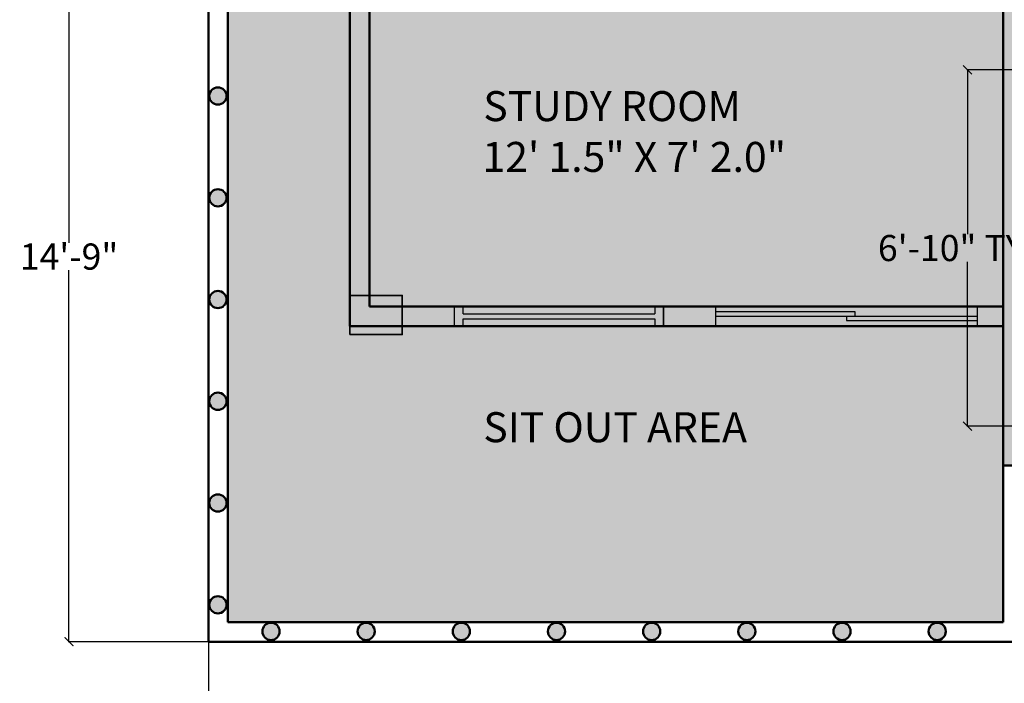
# Model space of a CAD drawing. Units: inches. Extents: x 528 to 2620, y -1066 to 798.
# Tile 21 of 41: x 981 to 1207, y 219 to 371. Entities that reach past the tile are written whole.
import ezdxf

# ---------------------------------------------------------------- set-up
doc = ezdxf.new("R2010")
doc.units = ezdxf.units.IN
doc.header["$MEASUREMENT"] = 0
for name, color, linetype, lineweight in [('A-ANNO-DIMS', 2, 'Continuous', 18), ('A-AREA-IDEN', 7, 'Continuous', 18), ('A-COLS', 1, 'Continuous', 35), ('A-Door', 2, 'Continuous', 25), ('A-GLAZ', 3, 'Continuous', 25), ('A-WALL', 7, 'Continuous', 50), ('A-WALL-PATT', 8, 'Continuous', 13)]:
    doc.layers.add(name, color=color, linetype=linetype, lineweight=lineweight)
doc.styles.get("Standard").update_dxf_attribs({"font": 'arial.ttf'})
doc.dimstyles.get("Standard").update_dxf_attribs({"dimtxt": 6, "dimasz": 2, "dimexe": 0.18, "dimexo": 0.0625, "dimgap": 0.09, "dimtad": 0, "dimtih": 1, "dimtoh": 1, "dimdec": 1, "dimzin": 0, "dimdsep": 46, "dimlunit": 3, "dimtxsty": 'Standard', "dimblk": 'ARCHTICK', "dimcen": 0.09, "dimadec": 0, "dimazin": 0, "dimtfac": 1, "dimtdec": 1, "dimtofl": 0, "dimtmove": 0, "dimatfit": 3, "dimfxl": 1, "dimtolj": 1, "dimtzin": 0, "dimarcsym": 0})

# ---------------------------------------------------------------- blocks, each defined once
blk = doc.blocks.new('_ArchTick')
at = {"color": 0, "linetype": 'ByBlock', "const_width": 0.15}
blk.add_lwpolyline([(-0.5, -0.5), (0.5, 0.5)], dxfattribs=at)
blk = doc.blocks.new('*D47')
at = {"layer": 'A-ANNO-DIMS', "color": 0, "lineweight": -2, "transparency": 16777216}
for p, q in [((1215.93, 359.77), (1198.62, 359.77)), ((1198.8, 359.77), (1198.8, 322)), ((1198.8, 277.92), (1198.8, 315.69)), ((1215.93, 277.92), (1198.62, 277.92))]:
    blk.add_line(p, q, dxfattribs=at)
at = {"layer": 'Defpoints', "color": 0, "transparency": 16777216}
for p in [(1216, 359.77), (1198.8, 277.92), (1216, 277.92)]:
    blk.add_point(p, dxfattribs=at)
at = {"layer": 'A-ANNO-DIMS', "color": 0, "lineweight": -2, "transparency": 16777216, "xscale": 2, "yscale": 2, "zscale": 2}
for p, rotation in [((1198.8, 359.77), 90), ((1198.8, 277.92), 270)]:
    blk.add_blockref('_ArchTick', p, dxfattribs=dict(at, rotation=rotation))
at = {"layer": 'A-ANNO-DIMS', "color": 0, "transparency": 16777216, "insert": (1198.8, 318.84), "char_height": 6, "attachment_point": 5}
blk.add_mtext('\\A1;6\'-10" TYP.', dxfattribs=at)
blk = doc.blocks.new('*D60')
at = {"layer": 'A-ANNO-DIMS', "color": 0, "lineweight": -2, "transparency": 16777216}
for p, q in [((1024.5, 228.36), (1024.5, 196.24)), ((1211.5, 228.36), (1211.5, 196.24)), ((1024.5, 196.42), (1107.88, 196.42)), ((1211.5, 196.42), (1128.11, 196.42))]:
    blk.add_line(p, q, dxfattribs=at)
at = {"layer": 'Defpoints', "color": 0, "transparency": 16777216}
for p in [(1024.5, 228.42), (1211.5, 228.42), (1211.5, 196.42)]:
    blk.add_point(p, dxfattribs=at)
at = {"layer": 'A-ANNO-DIMS', "color": 0, "lineweight": -2, "transparency": 16777216, "xscale": 2, "yscale": 2, "zscale": 2, "rotation": 180}
blk.add_blockref('_ArchTick', (1024.5, 196.42), dxfattribs=at)
at = {"layer": 'A-ANNO-DIMS', "color": 0, "lineweight": -2, "transparency": 16777216, "xscale": 2, "yscale": 2, "zscale": 2}
blk.add_blockref('_ArchTick', (1211.5, 196.42), dxfattribs=at)
at = {"layer": 'A-ANNO-DIMS', "color": 0, "transparency": 16777216, "insert": (1118, 196.42), "char_height": 6, "attachment_point": 5}
blk.add_mtext('\\A1;15\'-7"', dxfattribs=at)
blk = doc.blocks.new('*D64')
at = {"layer": 'A-ANNO-DIMS', "color": 0, "lineweight": -2, "transparency": 16777216}
for p, q in [((1024.43, 405.34), (992.32, 405.34)), ((992.5, 405.34), (992.5, 320.03)), ((992.5, 228.42), (992.5, 313.73)), ((1024.43, 228.42), (992.32, 228.42))]:
    blk.add_line(p, q, dxfattribs=at)
at = {"layer": 'Defpoints', "color": 0, "transparency": 16777216}
for p in [(1024.5, 405.34), (992.5, 228.42), (1024.5, 228.42)]:
    blk.add_point(p, dxfattribs=at)
at = {"layer": 'A-ANNO-DIMS', "color": 0, "lineweight": -2, "transparency": 16777216, "xscale": 2, "yscale": 2, "zscale": 2}
for p, rotation in [((992.5, 405.34), 90), ((992.5, 228.42), 270)]:
    blk.add_blockref('_ArchTick', p, dxfattribs=dict(at, rotation=rotation))
at = {"layer": 'A-ANNO-DIMS', "color": 0, "transparency": 16777216, "insert": (992.5, 316.88), "char_height": 6, "attachment_point": 5}
blk.add_mtext('\\A1;14\'-9"', dxfattribs=at)

msp = doc.modelspace()

# ---------------------------------------------------------------- hatches: boundary and pattern name
at = {"layer": 'A-COLS', "transparency": 33554687}
h = msp.add_hatch(color=256, dxfattribs=at)
h.dxf.hatch_style = 1
h.paths.add_polyline_path([(1057, 307.96), (1057, 298.96), (1069, 298.96), (1069, 307.96)])
at = {"layer": 'A-Door', "transparency": 33554687}
h = msp.add_hatch(color=256, dxfattribs=at)
h.dxf.hatch_style = 1
h.paths.add_polyline_path([(1201, 305.42), (1141, 305.42), (1141, 304.19), (1173.04, 304.19), (1173.04, 303.17), (1201, 303.17)])
h.paths.add_polyline_path([(1201, 302.21), (1171, 302.21), (1171, 303.17), (1141, 303.17), (1141, 300.92), (1201, 300.92)])
h = msp.add_hatch(color=256, dxfattribs=at)
h.dxf.hatch_style = 1
h.paths.add_polyline_path([(1201, 303.17), (1173.04, 303.17), (1171, 303.17), (1171, 302.21), (1201, 302.21)])
h.paths.add_polyline_path([(1173.04, 304.19), (1141, 304.19), (1141, 303.17), (1171, 303.17), (1173.04, 303.17)])
at = {"layer": 'A-GLAZ', "transparency": 33554687}
h = msp.add_hatch(color=256, dxfattribs=at)
h.dxf.hatch_style = 1
h.paths.add_polyline_path([(1061.5, 391.42), (1057, 391.42), (1057, 307.96), (1061.5, 307.96)])
h.paths.add_polyline_path([(1081, 305.42), (1069, 305.42), (1069, 300.92), (1081, 300.92)])
h.paths.add_polyline_path([(1141, 305.42), (1129, 305.42), (1129, 300.92), (1141, 300.92)])
h.paths.add_polyline_path([(1207, 305.42), (1201, 305.42), (1201, 300.92), (1207, 300.92)])
h = msp.add_hatch(color=256, dxfattribs=at)
h.dxf.hatch_style = 1
h.paths.add_polyline_path([(1129, 305.42), (1127, 305.42), (1127, 303.75), (1083, 303.75), (1083, 305.42), (1081, 305.42), (1081, 300.92), (1083, 300.92), (1083, 302.6), (1127, 302.6), (1127, 300.92), (1129, 300.92)])
h = msp.add_hatch(color=256, dxfattribs=at)
h.dxf.hatch_style = 1
h.paths.add_polyline_path([(1127, 305.42), (1083, 305.42), (1083, 303.75), (1127, 303.75)])
h.paths.add_polyline_path([(1127, 302.6), (1083, 302.6), (1083, 300.92), (1127, 300.92)])
at = {"layer": 'A-WALL-PATT', "transparency": 33554521}
h = msp.add_hatch(color=256, dxfattribs=at)
h.dxf.hatch_style = 1
h.paths.add_polyline_path([(1066, 709.92), (1114.5, 709.92), (1114.5, 718.92), (1057, 718.92), (1057, 667.92), (1066, 667.92)])
h.paths.add_polyline_path([(1227.5, 718.92), (1162.5, 718.92), (1162.5, 709.92), (1211, 709.92), (1211, 577.92), (1205.42, 577.92), (1205.5, 573.42), (1211, 573.42), (1211, 567.42), (1215.5, 567.42), (1215.5, 669.42), (1268, 669.42), (1268, 675.92), (1263.5, 675.92), (1263.5, 673.92), (1215.5, 673.92), (1215.5, 709.92), (1227.5, 709.92)])
h.paths.add_polyline_path([(1345, 718.92), (1316, 718.92), (1316, 709.92), (1336, 709.92), (1336, 641.67), (1345, 641.67)])
h.paths.add_polyline_path([(1066, 619.92), (1057, 619.92), (1057, 561.42), (1066, 561.42), (1066, 573.42), (1161, 573.42), (1161, 569.42), (1165.5, 569.42), (1165.5, 577.92), (1066, 577.92)])
h.paths.add_polyline_path([(1216, 391.42), (1216, 400.42), (1207, 400.42), (1201, 400.42), (1201, 397.42), (1201, 391.42), (1207, 391.42), (1207, 268.92), (1252, 268.92), (1252, 277.92), (1216, 277.92), (1216, 359.77)])
h.paths.add_polyline_path([(1345, 395.92), (1336, 395.92), (1288, 395.92), (1288, 391.42), (1336, 391.42), (1336, 277.92), (1300, 277.92), (1300, 268.92), (1345, 268.92)])
h.paths.add_polyline_path([(1345, 593.67), (1336, 593.67), (1336, 525.42), (1215.5, 525.42), (1215.5, 527.17), (1211, 527.17), (1211, 520.92), (1336, 520.92), (1336, 443.92), (1345, 443.92)])
h.paths.add_polyline_path([(1066, 520.92), (1165.5, 520.92), (1165.5, 545.42), (1161, 545.42), (1161, 525.42), (1066, 525.42), (1066, 537.42), (1057, 537.42), (1057, 484.67), (1066, 484.67)])
h.paths.add_polyline_path([(1066, 436.67), (1057, 436.67), (1057, 391.42), (1085.5, 391.42), (1085.5, 400.42), (1066, 400.42)])
h.paths.add_polyline_path([(1153, 397.42), (1153, 400.42), (1133.5, 400.42), (1133.5, 391.42), (1153, 391.42)])
at = {"layer": 'A-WALL-PATT', "transparency": 33554536}
h = msp.add_hatch(color=256, dxfattribs=at)
h.dxf.hatch_style = 1
h.paths.add_polyline_path([(1336, 709.92), (1268, 709.92), (1268, 699.92), (1266.75, 699.92), (1266.75, 675.92), (1268, 675.92), (1268, 669.42), (1215.5, 669.42), (1215.5, 567.17), (1217, 567.17), (1257, 567.17), (1257, 565.42), (1256.96, 565.42, -0.401453), (1217, 527.17), (1215.5, 527.17), (1215.5, 525.42), (1336, 525.42)], flags=17)
h.paths.add_polyline_path([(1285.03, 635.93), (1285.23, 636.13), (1285.67, 636.26), (1286.21, 636.02), (1286.98, 636.08), (1332.98, 636.08), (1333.36, 636.22), (1333.82, 636.08), (1334.11, 635.71), (1334.11, 635.3), (1333.91, 634.86), (1333.82, 634.83), (1333.82, 592.74), (1333.97, 592.6), (1334.11, 592.29), (1334.11, 591.88), (1333.82, 591.51), (1333.36, 591.37), (1332.98, 591.51), (1332.64, 591.79), (1332.64, 591.51), (1286.98, 591.51), (1286.17, 591.67), (1286.07, 591.57), (1285.68, 591.37), (1285.23, 591.51), (1285.03, 591.71), (1284.83, 592.1), (1284.98, 592.54), (1285.13, 592.69), (1285.13, 634.95), (1284.98, 635.1), (1284.83, 635.54)], flags=16)
h.paths.add_polyline_path([(1285.03, 635.93), (1285.23, 636.13), (1285.67, 636.26), (1286.21, 636.02), (1286.98, 636.08), (1332.98, 636.08), (1333.36, 636.22), (1333.82, 636.08), (1334.11, 635.71), (1334.11, 635.3), (1333.97, 634.99), (1333.82, 634.85), (1333.82, 592.74), (1333.97, 592.6), (1334.11, 592.29), (1334.11, 591.88), (1333.82, 591.51), (1333.36, 591.37), (1332.98, 591.51), (1332.64, 591.79), (1332.64, 592.25), (1332.64, 635.35), (1332.64, 635.8), (1332.98, 636.08), (1312.23, 636.08), (1311.1, 635.48), (1310.63, 635.48), (1310.43, 635.23), (1309.94, 635.1), (1309.7, 634.99), (1309.06, 634.76), (1308.71, 634.61), (1308.32, 634.61), (1307.75, 634.36), (1307.11, 634.27), (1307.01, 634.11), (1306.77, 634.02), (1307.25, 633.28), (1306.87, 633.04), (1306.77, 632.88), (1306.37, 632.64), (1306.03, 632.55), (1305.54, 632.41), (1315.47, 618.49), (1316.32, 619.39), (1312.77, 622.86), (1319.62, 630.11), (1320.07, 629.68), (1320.11, 630), (1320.28, 630.6), (1320.53, 631.18), (1320.53, 632.01), (1320.26, 632.55), (1320.11, 633.13), (1320.06, 633.73), (1320.63, 634.02), (1321.22, 634.16), (1321.86, 634.11), (1322.45, 633.91), (1322.99, 633.62), (1324.1, 633.62), (1324.64, 633.91), (1325.23, 634.07), (1325.87, 634.07), (1326.43, 633.91), (1326.98, 633.62), (1328.35, 633.62), (1328.9, 633.91), (1329.49, 634.11), (1330.1, 634.16), (1330.69, 634.02), (1331.28, 633.73), (1331.23, 633.13), (1331.09, 632.55), (1330.79, 632.01), (1330.79, 631.18), (1331.04, 630.6), (1331.23, 630), (1331.28, 629.41), (1331.19, 628.79), (1331.04, 628.18), (1330.79, 627.6), (1330.79, 626.77), (1331.04, 626.19), (1331.23, 625.59), (1331.28, 625.01), (1331.19, 624.38), (1331.04, 623.78), (1330.79, 623.24), (1330.79, 622.37), (1331.04, 621.83), (1331.23, 621.25), (1331.28, 620.6), (1331.19, 619.97), (1331.04, 619.37), (1330.79, 618.83), (1330.79, 617.96), (1331.09, 617.42), (1331.23, 616.88), (1331.28, 616.23), (1331.28, 615.52), (1330.69, 615.27), (1330.1, 615.12), (1329.49, 615.12), (1328.9, 615.32), (1328.35, 615.65), (1326.98, 615.65), (1326.43, 615.32), (1325.87, 615.16), (1325.23, 615.16), (1324.64, 615.32), (1324.1, 615.65), (1323.24, 615.65), (1324.93, 614.04), (1322.98, 611.98), (1324.1, 611.98), (1324.64, 612.27), (1325.28, 612.43), (1325.87, 612.43), (1326.48, 612.27), (1327.03, 611.98), (1328.35, 611.98), (1328.9, 612.27), (1329.49, 612.48), (1330.1, 612.52), (1330.74, 612.39), (1331.28, 612.07), (1331.28, 611.36), (1331.28, 610.75), (1331.09, 610.17), (1330.79, 609.63), (1330.79, 608.81), (1331.09, 608.22), (1331.23, 607.62), (1331.28, 606.99), (1331.23, 606.41), (1331.09, 605.81), (1330.79, 605.22), (1330.79, 604.4), (1331.09, 603.81), (1331.23, 603.21), (1331.28, 602.63), (1331.23, 602), (1331.09, 601.4), (1330.79, 600.86), (1330.79, 599.99), (1331.09, 599.45), (1331.23, 598.87), (1331.28, 598.22), (1331.23, 597.59), (1331.09, 596.99), (1330.79, 596.45), (1330.79, 595.58), (1331.09, 595.04), (1331.28, 594.51), (1331.28, 593.86), (1330.74, 593.61), (1330.1, 593.48), (1329.49, 593.48), (1328.9, 593.68), (1328.35, 594.01), (1327.03, 594.01), (1326.48, 593.68), (1325.87, 593.52), (1325.28, 593.52), (1324.64, 593.68), (1324.1, 594.01), (1323.04, 594.01), (1322.5, 593.68), (1321.91, 593.48), (1321.27, 593.48), (1320.63, 593.61), (1320.11, 593.86), (1320.11, 594.51), (1320.28, 595.04), (1320.58, 595.58), (1320.58, 596.45), (1320.28, 596.99), (1320.16, 597.59), (1320.1, 598.01), (1319.62, 597.55), (1315.66, 601.73), (1312.23, 591.57), (1311.74, 591.66), (1311.59, 591.91), (1310.78, 592.4), (1309.55, 592.89), (1308.96, 592.89), (1308.71, 593.03), (1308.56, 593.14), (1307.75, 593.52), (1306.77, 593.61), (1307.25, 594.36), (1306.87, 594.6), (1306.37, 594.84), (1306.03, 595.09), (1305.54, 595.24), (1315.46, 609.35), (1310.93, 613.71), (1315.47, 618.49), (1305.54, 632.41), (1306.03, 632.55), (1306.37, 632.64), (1306.77, 632.88), (1306.87, 633.04), (1307.25, 633.28), (1306.77, 634.02), (1307.01, 634.11), (1307.11, 634.27), (1307.75, 634.36), (1308.32, 634.61), (1308.71, 634.61), (1309.06, 634.76), (1309.7, 634.99), (1309.94, 635.1), (1310.43, 635.23), (1310.63, 635.48), (1311.1, 635.48), (1312.23, 636.08), (1286.98, 636.08), (1286.22, 636.02), (1286.41, 635.44), (1286.21, 635.05), (1286.02, 634.85), (1285.87, 634.81), (1285.87, 592.84), (1286.15, 592.73), (1286.41, 592.19), (1286.23, 591.66), (1286.17, 591.67), (1286.07, 591.57), (1285.68, 591.37), (1285.23, 591.51), (1285.03, 591.71), (1284.83, 592.1), (1284.98, 592.54), (1285.13, 592.69), (1285.13, 634.95), (1284.98, 635.1), (1284.83, 635.54)], flags=0)
h.paths.add_polyline_path([(1322.5, 653.6), (1333.65, 653.6), (1333.65, 637.99), (1322.5, 637.99)], flags=16)
h.paths.add_polyline_path([(1323.62, 652.48), (1332.53, 652.48), (1332.53, 639.11), (1323.62, 639.11)], flags=0)
edge = h.paths.add_edge_path(flags=0)
edge.add_ellipse((1328.07, 645.79), major_axis=(2.24, 2.24), ratio=1, start_angle=405, end_angle=495, ccw=False)
edge.add_ellipse((1328.07, 645.79), major_axis=(2.24, 2.24), ratio=1, start_angle=675, end_angle=765, ccw=False)
edge.add_ellipse((1328.07, 645.79), major_axis=(2.24, 2.24), ratio=1, start_angle=585, end_angle=675, ccw=False)
edge.add_ellipse((1328.07, 645.79), major_axis=(2.24, 2.24), ratio=1, start_angle=495, end_angle=585, ccw=False)
h.paths.add_polyline_path([(1320.58, 628.39), (1320.33, 628.01), (1320.61, 628.55)], flags=0)
h.paths.add_polyline_path([(1317.89, 604.89), (1318.78, 604.64), (1319.76, 604.28), (1318.88, 604.53)], flags=0)
h.paths.add_polyline_path([(1320.33, 599.65), (1320.58, 599.25), (1320.58, 599.16)], flags=0)
h.paths.add_polyline_path([(1322.5, 589.6), (1333.65, 589.6), (1333.65, 573.99), (1322.5, 573.99)], flags=16)
h.paths.add_polyline_path([(1323.62, 588.48), (1332.53, 588.48), (1332.53, 575.11), (1323.62, 575.11)], flags=0)
edge = h.paths.add_edge_path(flags=0)
edge.add_ellipse((1328.07, 581.8), major_axis=(-2.24, 2.24), ratio=1, start_angle=-45, end_angle=45, ccw=False)
edge.add_ellipse((1328.07, 581.8), major_axis=(-2.24, 2.24), ratio=1, start_angle=-135, end_angle=-45, ccw=False)
edge.add_ellipse((1328.07, 581.8), major_axis=(-2.24, 2.24), ratio=1, start_angle=135, end_angle=-135, ccw=False)
edge.add_ellipse((1328.07, 581.8), major_axis=(-2.24, 2.24), ratio=1, start_angle=45, end_angle=135, ccw=False)
h.paths.add_polyline_path([(1264.75, 699.92), (1263.5, 699.92), (1263.5, 709.92), (1215.5, 709.92), (1215.5, 673.92), (1263.5, 673.92), (1263.5, 675.92), (1264.75, 675.92)], flags=16)
h.paths.add_polyline_path([(1162.19, 569.42), (1161, 569.42), (1161, 573.42), (1066, 573.42), (1066, 525.42), (1161, 525.42), (1161, 545.42), (1162.19, 545.42)])
h.paths.add_polyline_path([(1256.96, 565.42), (1257, 565.42), (1257, 567.17), (1217, 567.17), (1215.5, 567.17), (1215.5, 567.42), (1211, 567.42), (1211, 573.42), (1205.5, 573.42), (1205.42, 577.92), (1211, 577.92), (1211, 709.92), (1066, 709.92), (1066, 577.92), (1165.5, 577.92), (1165.5, 569.42), (1164.19, 569.42), (1164.19, 545.42), (1165.5, 545.42), (1165.5, 520.92), (1153, 520.92), (1153, 484.92), (1102, 484.92), (1102, 436.42), (1153, 436.42), (1153, 400.42), (1153, 391.42), (1201, 391.42), (1201, 400.42), (1207, 400.42), (1216, 400.42), (1216, 391.42), (1216, 277.92), (1336, 277.92), (1336, 391.42), (1288, 391.42), (1288, 395.92), (1336, 395.92), (1336, 443.92), (1336, 520.92), (1211, 520.92), (1211, 527.17), (1215.5, 527.17), (1217, 527.17, 0.401453)])
h.paths.add_polyline_path([(1167.25, 579.42), (1165.5, 579.42), (1165.5, 619.42), (1167.25, 619.42)], flags=16)
h.paths.add_polyline_path([(1227.97, 501.56), (1236.36, 502.03), (1236.36, 492.55), (1227.97, 493.02, -0.254069)], flags=16)
h.paths.add_polyline_path([(1243.34, 515.69, -0.254069), (1251.88, 515.69), (1252.35, 507.3), (1242.87, 507.3)], flags=16)
h.paths.add_polyline_path([(1239.18, 504.68), (1256.03, 504.68), (1256.03, 479.42), (1239.18, 479.42)], flags=16)
h.paths.add_polyline_path([(1227.97, 489.6), (1236.36, 490.07), (1236.36, 480.59), (1227.97, 481.06, -0.254069)], flags=16)
h.paths.add_polyline_path([(1197.2, 624.04), (1197.2, 639.64), (1208.35, 639.64), (1208.35, 624.04)], flags=16)
h.paths.add_polyline_path([(1198.32, 625.15), (1198.32, 638.53), (1207.23, 638.53), (1207.23, 625.15)], flags=0)
h.paths.add_polyline_path([(1258.85, 502.03), (1267.25, 501.56, -0.254069), (1267.25, 493.02), (1258.85, 492.55)], flags=16)
h.paths.add_polyline_path([(1271.59, 519.66), (1333.67, 519.66), (1333.67, 451.59), (1319.09, 451.59), (1319.09, 505.07), (1288.09, 505.07), (1284.45, 505.07, -0.883215), (1270.68, 514.19), (1270.68, 518.75, -0.414214)], flags=16)
h.paths.add_polyline_path([(1331.85, 517.83), (1331.85, 453.42), (1328.2, 453.42), (1328.2, 505.07), (1298.42, 505.07), (1298.42, 514.19), (1288.09, 514.19), (1288.09, 517.83)], flags=0)
h.paths.add_polyline_path([(1242.87, 476.8), (1252.35, 476.8), (1251.88, 468.41, -0.254069), (1243.34, 468.41)], flags=16)
h.paths.add_polyline_path([(1258.85, 490.07), (1267.25, 489.6, -0.254069), (1267.25, 481.06), (1258.85, 480.59)], flags=16)
h.paths.add_polyline_path([(1161.68, 641.55), (1160.87, 641.72), (1160.77, 641.62), (1160.38, 641.41), (1159.93, 641.55), (1159.73, 641.75), (1159.53, 642.14), (1159.68, 642.58), (1159.83, 642.73), (1159.83, 684.99), (1159.68, 685.14), (1159.53, 685.58), (1159.73, 685.97), (1159.93, 686.17), (1160.37, 686.31), (1160.91, 686.06), (1161.68, 686.13), (1207.68, 686.13), (1208.06, 686.27), (1208.52, 686.13), (1208.81, 685.76), (1208.81, 685.34), (1208.61, 684.9), (1208.52, 684.87), (1208.52, 642.78), (1208.67, 642.65), (1208.88, 642.2), (1208.72, 641.8), (1208.52, 641.55), (1208.06, 641.41), (1207.68, 641.55), (1207.34, 641.83), (1207.34, 641.55)], flags=16)
h.paths.add_polyline_path([(1186.93, 641.62), (1186.44, 641.71), (1186.29, 641.95), (1185.48, 642.45), (1184.25, 642.94), (1183.66, 642.94), (1183.41, 643.07), (1183.26, 643.18), (1182.45, 643.57), (1181.47, 643.65), (1181.95, 644.4), (1181.57, 644.64), (1181.07, 644.89), (1180.73, 645.13), (1180.24, 645.29), (1190.16, 659.4), (1185.63, 663.75), (1190.17, 668.54), (1180.24, 682.46), (1180.73, 682.59), (1181.07, 682.68), (1181.47, 682.93), (1181.57, 683.08), (1181.95, 683.33), (1181.47, 684.07), (1181.71, 684.16), (1181.81, 684.31), (1182.45, 684.4), (1183.02, 684.65), (1183.41, 684.65), (1183.76, 684.81), (1184.4, 685.03), (1184.64, 685.14), (1185.13, 685.28), (1185.33, 685.52), (1185.8, 685.52), (1186.93, 686.13), (1161.68, 686.13), (1160.92, 686.06), (1161.11, 685.49), (1160.91, 685.1), (1160.72, 684.9), (1160.57, 684.85), (1160.57, 642.88), (1160.85, 642.77), (1161.11, 642.23), (1160.93, 641.7), (1160.87, 641.72), (1160.77, 641.62), (1160.38, 641.41), (1159.93, 641.55), (1159.73, 641.75), (1159.53, 642.14), (1159.68, 642.58), (1159.83, 642.73), (1159.83, 684.99), (1159.68, 685.14), (1159.53, 685.58), (1159.73, 685.97), (1159.93, 686.17), (1160.37, 686.31), (1160.91, 686.06), (1161.68, 686.13), (1207.68, 686.13), (1208.06, 686.27), (1208.52, 686.13), (1208.81, 685.76), (1208.81, 685.34), (1208.67, 685.03), (1208.52, 684.9), (1208.52, 642.78), (1208.67, 642.65), (1208.88, 642.2), (1208.72, 641.8), (1208.52, 641.55), (1208.06, 641.41), (1207.68, 641.55), (1207.34, 641.83), (1207.34, 642.29), (1207.34, 685.39), (1207.34, 685.85), (1207.68, 686.13), (1186.93, 686.13), (1185.8, 685.52), (1185.33, 685.52), (1185.13, 685.28), (1184.64, 685.14), (1184.4, 685.03), (1183.76, 684.81), (1183.41, 684.65), (1183.02, 684.65), (1182.45, 684.4), (1181.81, 684.31), (1181.71, 684.16), (1181.47, 684.07), (1181.95, 683.33), (1181.57, 683.08), (1181.47, 682.93), (1181.07, 682.68), (1180.73, 682.59), (1180.24, 682.46), (1190.17, 668.54), (1191.02, 669.43), (1187.47, 672.9), (1194.32, 680.15), (1194.77, 679.72), (1194.81, 680.04), (1194.98, 680.65), (1195.23, 681.23), (1195.23, 682.05), (1194.96, 682.59), (1194.81, 683.17), (1194.76, 683.78), (1195.33, 684.07), (1195.92, 684.2), (1196.56, 684.16), (1197.15, 683.96), (1197.69, 683.67), (1198.8, 683.67), (1199.34, 683.96), (1199.93, 684.11), (1200.57, 684.11), (1201.13, 683.96), (1201.68, 683.67), (1203.05, 683.67), (1203.6, 683.96), (1204.19, 684.16), (1204.8, 684.2), (1205.39, 684.07), (1205.98, 683.78), (1205.93, 683.17), (1205.79, 682.59), (1205.49, 682.05), (1205.49, 681.23), (1205.74, 680.65), (1205.93, 680.04), (1205.98, 679.46), (1205.89, 678.83), (1205.74, 678.23), (1205.49, 677.65), (1205.49, 676.82), (1205.74, 676.24), (1205.93, 675.63), (1205.98, 675.05), (1205.89, 674.42), (1205.74, 673.82), (1205.49, 673.28), (1205.49, 672.41), (1205.74, 671.87), (1205.93, 671.29), (1205.98, 670.64), (1205.89, 670.02), (1205.74, 669.41), (1205.49, 668.87), (1205.49, 668), (1205.79, 667.46), (1205.93, 666.93), (1205.98, 666.28), (1205.98, 665.56), (1205.39, 665.32), (1204.8, 665.16), (1204.19, 665.16), (1203.6, 665.36), (1203.05, 665.7), (1201.68, 665.7), (1201.13, 665.36), (1200.57, 665.2), (1199.93, 665.2), (1199.34, 665.36), (1198.8, 665.7), (1197.94, 665.7), (1199.63, 664.09), (1197.68, 662.03), (1198.8, 662.03), (1199.34, 662.32), (1199.98, 662.47), (1200.57, 662.47), (1201.18, 662.32), (1201.73, 662.03), (1203.05, 662.03), (1203.6, 662.32), (1204.19, 662.52), (1204.8, 662.56), (1205.44, 662.43), (1205.98, 662.12), (1205.98, 661.4), (1205.98, 660.8), (1205.79, 660.21), (1205.49, 659.68), (1205.49, 658.85), (1205.79, 658.27), (1205.93, 657.66), (1205.98, 657.04), (1205.93, 656.45), (1205.79, 655.85), (1205.49, 655.27), (1205.49, 654.44), (1205.79, 653.86), (1205.93, 653.25), (1205.98, 652.67), (1205.93, 652.05), (1205.79, 651.44), (1205.49, 650.91), (1205.49, 650.03), (1205.79, 649.5), (1205.93, 648.91), (1205.98, 648.26), (1205.93, 647.64), (1205.79, 647.03), (1205.49, 646.5), (1205.49, 645.62), (1205.79, 645.09), (1205.98, 644.55), (1205.98, 643.9), (1205.44, 643.65), (1204.8, 643.52), (1204.19, 643.52), (1203.6, 643.72), (1203.05, 644.06), (1201.73, 644.06), (1201.18, 643.72), (1200.57, 643.57), (1199.98, 643.57), (1199.34, 643.72), (1198.8, 644.06), (1197.74, 644.06), (1197.2, 643.72), (1196.61, 643.52), (1195.97, 643.52), (1195.33, 643.65), (1194.81, 643.9), (1194.81, 644.55), (1194.98, 645.09), (1195.28, 645.62), (1195.28, 646.5), (1194.98, 647.03), (1194.86, 647.64), (1194.8, 648.06), (1194.32, 647.59), (1190.36, 651.77)], flags=16)
h.paths.add_polyline_path([(1195.28, 649.2), (1195.03, 649.7), (1195.28, 649.29)], flags=0)
h.paths.add_polyline_path([(1194.46, 654.33), (1193.58, 654.58), (1192.59, 654.93), (1193.48, 654.69)], flags=0)
h.paths.add_polyline_path([(1195.28, 678.43), (1195.03, 678.05), (1195.31, 678.59)], flags=0)
h.paths.add_polyline_path([(1197.2, 688.04), (1197.2, 703.64), (1208.35, 703.64), (1208.35, 688.04)], flags=16)
h.paths.add_polyline_path([(1198.32, 689.15), (1198.32, 702.53), (1207.23, 702.53), (1207.23, 689.15)], flags=0)
h.paths.add_polyline_path([(1217.1, 329.02), (1230.65, 329.02), (1230.65, 315.47), (1217.1, 315.47)], flags=16)
h.paths.add_polyline_path([(1223.87, 322.24), (1227.26, 322.24), (1227.26, 321.32, -0.414214), (1229.73, 318.86, -1), (1224.8, 318.86), (1223.87, 318.86)], flags=0)
h.paths.add_polyline_path([(1222.11, 325.63, -1), (1218.86, 325.63, -1)], flags=0)
h.paths.add_polyline_path([(1228.25, 325.63, -1), (1226.28, 325.63, -1)], flags=0)
h.paths.add_polyline_path([(1221.53, 318.86, -1), (1219.44, 318.86, -1)], flags=0)
h.paths.add_polyline_path([(1299.15, 293.73), (1299.15, 278.54), (1271.23, 278.54), (1271.23, 293.73)], flags=16)
h.paths.add_polyline_path([(1259.69, 292.21), (1270.62, 292.21, -1), (1270.62, 291.6), (1259.69, 291.6, -1)], flags=16)
h.paths.add_polyline_path([(1259.69, 291.3), (1270.62, 291.3, -1), (1270.62, 290.69), (1259.69, 290.69, -1)], flags=16)
h.paths.add_polyline_path([(1259.69, 290.39), (1270.62, 290.39, -1), (1270.62, 289.78), (1259.69, 289.78, -1)], flags=16)
h.paths.add_polyline_path([(1259.69, 289.48), (1270.62, 289.48, -1), (1270.62, 288.87), (1259.69, 288.87, -1)], flags=16)
h.paths.add_polyline_path([(1259.69, 288.57), (1270.62, 288.57, -1), (1270.62, 287.96), (1259.69, 287.96, -1)], flags=16)
h.paths.add_polyline_path([(1274.41, 292.38), (1283.25, 292.38, -0.414214), (1285.07, 290.56), (1285.07, 283.64, -0.414214), (1283.25, 281.82), (1277.72, 281.82), (1278.67, 280.87, -0.57735), (1279.38, 280.16), (1279.44, 280.11, -1), (1279.03, 279.7), (1278.97, 279.75, -0.57735), (1278.26, 280.46), (1276.9, 281.82), (1274.41, 281.82, -0.414214), (1272.58, 283.64), (1272.58, 290.56, -0.414214)], flags=0)
h.paths.add_polyline_path([(1259.69, 287.65), (1270.62, 287.65, -1), (1270.62, 287.05), (1259.69, 287.05, -1)], flags=16)
h.paths.add_polyline_path([(1259.69, 286.74), (1270.62, 286.74, -1), (1270.62, 286.14), (1259.69, 286.14, -1)], flags=16)
h.paths.add_polyline_path([(1259.69, 285.83), (1270.62, 285.83, -1), (1270.62, 285.22), (1259.69, 285.22, -1)], flags=16)
h.paths.add_polyline_path([(1259.69, 284.92), (1270.62, 284.92, -1), (1270.62, 284.31), (1259.69, 284.31, -1)], flags=16)
h.paths.add_polyline_path([(1259.69, 284.01), (1270.62, 284.01, -1), (1270.62, 283.4), (1259.69, 283.4, -1)], flags=16)
h.paths.add_polyline_path([(1287.82, 292.38), (1296.67, 292.38, -0.414214), (1298.49, 290.56), (1298.49, 283.64, -0.414214), (1296.67, 281.82), (1291.14, 281.82), (1292.09, 280.87, -0.57735), (1292.8, 280.16), (1292.85, 280.11, -1), (1292.44, 279.7), (1292.39, 279.75, -0.57735), (1291.68, 280.46), (1290.32, 281.82), (1287.82, 281.82, -0.414214), (1286, 283.64), (1286, 290.56, -0.414214)], flags=0)
h.paths.add_polyline_path([(1259.69, 283.1), (1270.62, 283.1, -1), (1270.62, 282.49), (1259.69, 282.49, -1)], flags=16)
h.paths.add_polyline_path([(1279.94, 287.61, -1), (1278.01, 287.61, -1)], flags=0)
h.paths.add_polyline_path([(1259.69, 282.19), (1270.62, 282.19, -1), (1270.62, 281.58), (1259.69, 281.58, -1)], flags=16)
h.paths.add_polyline_path([(1259.69, 281.27), (1270.62, 281.27, -1), (1270.62, 280.67), (1259.69, 280.67, -1)], flags=16)
h.paths.add_polyline_path([(1275.16, 284.17, -1), (1274.77, 284.17, -1)], flags=0)
h.paths.add_polyline_path([(1293.36, 287.61, -1), (1291.43, 287.61, -1)], flags=0)
h.paths.add_polyline_path([(1275.14, 280.5), (1276.33, 280.5, -5.828427), (1276.33, 280.12), (1275.14, 280.12, -1)], flags=0)
h.paths.add_polyline_path([(1288.57, 284.17, -1), (1288.19, 284.17, -1)], flags=0)
h.paths.add_polyline_path([(1281.31, 280.5), (1282.5, 280.5, -1), (1282.5, 280.12), (1281.31, 280.12, -5.828427)], flags=0)
h.paths.add_polyline_path([(1288.56, 280.5), (1289.75, 280.5, -5.828427), (1289.75, 280.12), (1288.56, 280.12, -1)], flags=0)
h.paths.add_polyline_path([(1294.73, 280.5), (1295.92, 280.5, -1), (1295.92, 280.12), (1294.73, 280.12, -5.828427)], flags=0)
h.paths.add_polyline_path([(1207, 391.42), (1201, 391.42), (1061.5, 391.42), (1061.5, 307.96), (1069, 307.96), (1069, 305.42), (1207, 305.42)])
h = msp.add_hatch(color=256, dxfattribs=at)
h.dxf.hatch_style = 1
h.paths.add_polyline_path([(1207, 300.92), (1069, 300.92), (1069, 298.96), (1057, 298.96), (1057, 307.96), (1057, 391.42), (1057, 400.84), (1029, 400.84), (1029, 232.92), (1207, 232.92), (1207, 268.92)])
at = {"layer": 'A-WALL-PATT', "transparency": 33554687}
h = msp.add_hatch(color=256, dxfattribs=at)
h.dxf.hatch_style = 1
h.paths.add_polyline_path([(1024.71, 353.75, 1), (1028.67, 353.75, 1)])
h = msp.add_hatch(color=256, dxfattribs=at)
h.dxf.hatch_style = 1
h.paths.add_polyline_path([(1024.71, 330.38, 1), (1028.67, 330.38, 1)])
h = msp.add_hatch(color=256, dxfattribs=at)
h.dxf.hatch_style = 1
h.paths.add_polyline_path([(1024.71, 307.01, 1), (1028.67, 307.01, 1)])
h = msp.add_hatch(color=256, dxfattribs=at)
h.dxf.hatch_style = 1
h.paths.add_polyline_path([(1024.71, 283.64, 1), (1028.67, 283.64, 1)])
h = msp.add_hatch(color=256, dxfattribs=at)
h.dxf.hatch_style = 1
h.paths.add_polyline_path([(1024.71, 260.27, 1), (1028.67, 260.27, 1)])
h = msp.add_hatch(color=256, dxfattribs=at)
h.dxf.hatch_style = 1
h.paths.add_polyline_path([(1024.71, 236.89, 1), (1028.67, 236.89, 1)])
h = msp.add_hatch(color=256, dxfattribs=at)
h.dxf.hatch_style = 1
h.paths.add_polyline_path([(1036.89, 230.78, 1), (1040.86, 230.78, 1)])
h = msp.add_hatch(color=256, dxfattribs=at)
h.dxf.hatch_style = 1
h.paths.add_polyline_path([(1058.74, 230.78, 1), (1062.71, 230.78, 1)])
h = msp.add_hatch(color=256, dxfattribs=at)
h.dxf.hatch_style = 1
h.paths.add_polyline_path([(1080.6, 230.78, 1), (1084.56, 230.78, 1)])
h = msp.add_hatch(color=256, dxfattribs=at)
h.dxf.hatch_style = 1
h.paths.add_polyline_path([(1102.45, 230.78, 1), (1106.41, 230.78, 1)])
h = msp.add_hatch(color=256, dxfattribs=at)
h.dxf.hatch_style = 1
h.paths.add_polyline_path([(1124.3, 230.78, 1), (1128.27, 230.78, 1)])
h = msp.add_hatch(color=256, dxfattribs=at)
h.dxf.hatch_style = 1
h.paths.add_polyline_path([(1146.15, 230.78, 1), (1150.12, 230.78, 1)])
h = msp.add_hatch(color=256, dxfattribs=at)
h.dxf.hatch_style = 1
h.paths.add_polyline_path([(1168, 230.78, 1), (1171.97, 230.78, 1)])
h = msp.add_hatch(color=256, dxfattribs=at)
h.dxf.hatch_style = 1
h.paths.add_polyline_path([(1189.85, 230.78, 1), (1193.82, 230.78, 1)])

# ---------------------------------------------------------------- linework, layer by layer
at = {"layer": 'A-COLS'}
msp.add_lwpolyline([(1057, 298.96), (1057, 307.96), (1069, 307.96), (1069, 298.96)], close=True, dxfattribs=at)
at = {"layer": 'A-Door'}
for p, q in [((1201, 305.42), (1201, 300.92)), ((1173.04, 304.19), (1141, 304.19)), ((1141, 303.17), (1171, 303.17)), ((1171, 303.17), (1173.04, 303.17)), ((1171, 303.17), (1171, 302.21)), ((1173.04, 303.17), (1173.04, 304.19)), ((1173.04, 303.17), (1201, 303.17)), ((1171, 302.21), (1201, 302.21))]:
    msp.add_line(p, q, dxfattribs=at)
msp.add_lwpolyline([(1141, 305.42), (1201, 305.42), (1201, 300.92), (1141, 300.92)], close=True, dxfattribs=at)
at = {"layer": 'A-GLAZ'}
for p, q in [((1081, 305.42), (1129, 305.42)), ((1081, 300.92), (1081, 305.42)), ((1083, 303.75), (1083, 305.42)), ((1127, 305.42), (1127, 303.75)), ((1129, 305.42), (1129, 300.92)), ((1129, 300.92), (1129, 305.42)), ((1083, 303.75), (1127, 303.75)), ((1129, 300.92), (1081, 300.92)), ((1083, 300.92), (1083, 302.6)), ((1083, 302.6), (1127, 302.6)), ((1127, 302.6), (1127, 300.92))]:
    msp.add_line(p, q, dxfattribs=at)
at = {"layer": 'A-WALL'}
for p, q in [((1024.5, 405.34), (1024.5, 228.42)), ((1029, 400.84), (1029, 232.92)), ((1057, 391.42), (1057, 300.92)), ((1061.5, 391.42), (1061.5, 305.42)), ((1207, 268.92), (1207, 391.42)), ((1207, 391.42), (1207, 268.92)), ((1061.5, 305.42), (1207, 305.42)), ((1057, 300.92), (1207, 300.92)), ((1207, 268.92), (1345, 268.92)), ((1207, 268.92), (1207, 232.92)), ((1029, 232.92), (1207, 232.92)), ((1024.5, 228.42), (1211.5, 228.42))]:
    msp.add_line(p, q, dxfattribs=at)
for centre in [(1026.69, 353.75), (1026.69, 330.38), (1026.69, 307.01), (1026.69, 283.64), (1026.69, 260.27), (1026.69, 236.89), (1038.88, 230.78), (1060.73, 230.78), (1082.58, 230.78), (1104.43, 230.78), (1126.28, 230.78), (1148.13, 230.78), (1169.99, 230.78), (1191.84, 230.78)]:
    msp.add_circle(centre, 1.98, dxfattribs=at)

# ---------------------------------------------------------------- texts
at = {"layer": 'A-AREA-IDEN'}
for s, height, p in [('STUDY ROOM', 6.891, (1087.63, 347.99)), ('12\' 1.5" X 7\' 2.0"', 6.8907, (1087.44, 336.32)), ('SIT OUT AREA', 6.8907, (1087.63, 274.24))]:
    msp.add_text(s, height=height, dxfattribs=at).set_placement(p)

# ---------------------------------------------------------------- dimensions: what is measured, and where the dimension line sits
at = {"layer": 'A-ANNO-DIMS'}
dim = msp.add_linear_dim(base=(992.5, 228.42), p1=(1024.5, 405.34), p2=(1024.5, 228.42), angle=90, dimstyle='Standard', override={"dimdec": 1, "dimlfac": 1, "dimrnd": 0, "dimzin": 1, "dimdsep": 46, "dimlunit": 4, "dimfrac": 2}, dxfattribs=at)
dim.commit()
dim.dimension.update_dxf_attribs({"geometry": '*D64', "text_midpoint": (992.5, 316.88)})
dim = msp.add_linear_dim(base=(1198.805, 277.9223), p1=(1215.9964, 359.7668), p2=(1215.9964, 277.9223), angle=270, text='<> TYP.', dimstyle='Standard', override={"dimdec": 1, "dimrnd": 0, "dimzin": 1, "dimlunit": 4, "dimfrac": 2}, dxfattribs=at)
dim.commit()
dim.dimension.update_dxf_attribs({"geometry": '*D47', "text_midpoint": (1198.805, 318.8446)})
dim = msp.add_linear_dim(base=(1211.5, 196.42), p1=(1024.5, 228.42), p2=(1211.5, 228.42), dimstyle='Standard', override={"dimdec": 1, "dimlfac": 1, "dimrnd": 0, "dimzin": 1, "dimdsep": 46, "dimlunit": 4, "dimfrac": 2}, dxfattribs=at)
dim.commit()
dim.dimension.update_dxf_attribs({"geometry": '*D60', "text_midpoint": (1118, 196.42)})

doc.saveas('drawing.dxf')
